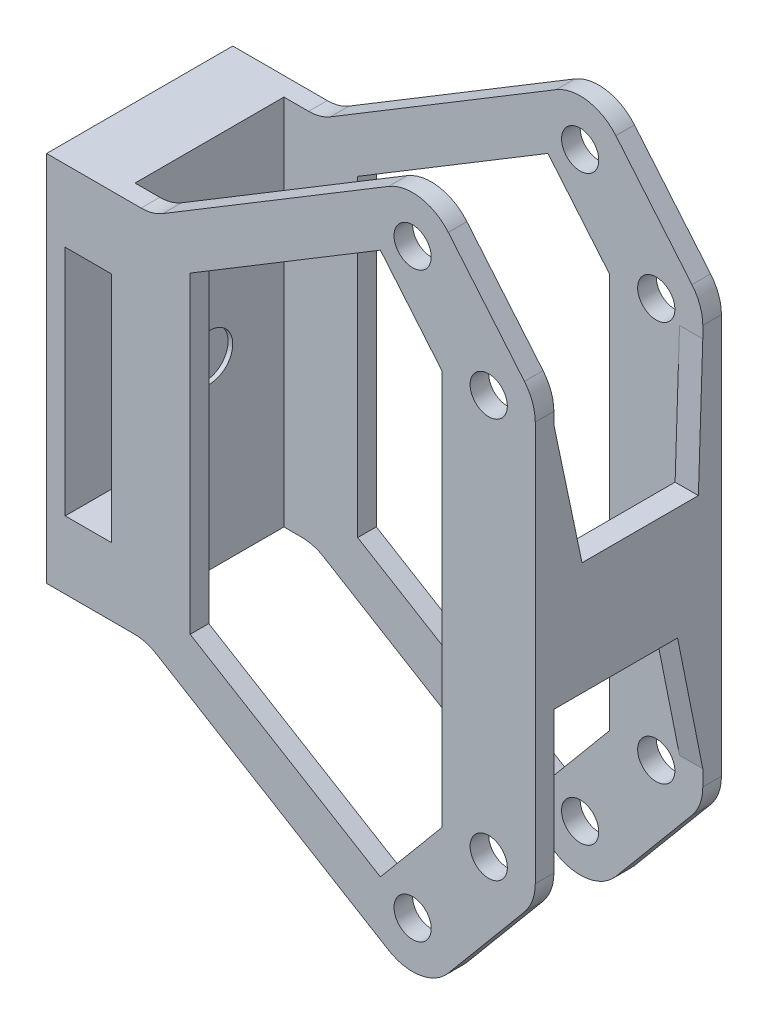
from build123d import *

# Parameters (mm, degrees)
BRACKET_PROFILE_SKETCH_R    = 4
BRACKET_PROFILE_SKETCH_W    = 10
BRACKET_PROFILE_SKETCH_H    = 50
BRACKET_BODY_DEPTH          = 20
SIDE_CUTOUT_DEPTH           = 151.958708937
SIDE_CUTOUT_DEPTH_BACK      = 151.958708937
SIDE_CUTOUT_SKETCH_W        = 85
SIDE_CUTOUT_SKETCH_H        = 32
INNER_WINDOW_CUT_DEPTH      = 130.155913531
INNER_WINDOW_CUT_DEPTH_BACK = 130.155913531
INNER_WINDOW_SKETCH_W       = 32
INNER_WINDOW_SKETCH_H       = 12.117592982
INNER_WINDOW_SKETCH_H_2     = 13.000486956
SIDE_OPENINGS_CUT_DEPTH     = 40
HOLE_10_SKETCH_R            = 5
THROUGH_HOLE_10_DEPTH       = 40
RECESS_24_SKETCH_R          = 12
RECESS_24X3_DEPTH           = 3


with BuildPart() as part:
    # Bracket Profile Sketch → Bracket Body (new, symmetric)
    with BuildSketch(Plane.XY):
        with BuildLine():
            Line((18.112706939, 41.738939357), (66.624129095, 71.058341812))
            ThreePointArc((66.624129095, 71.058341812), (73.442433942, 72.363637042), (79.467576157, 68.915342115))
            Line((79.467576157, 68.915342115), (95.817576157, 49.365342115))
            ThreePointArc((95.817576157, 49.365342115), (97.546351125, 46.362517955), (98.146631916, 42.95))
            Line((98.146631916, 42.95), (98.146631916, -42.95))
            ThreePointArc((98.146631916, -42.95), (97.546351125, -46.362517955), (95.817576157, -49.365342115))
            Line((95.817576157, -49.365342115), (79.467576157, -68.915342115))
            ThreePointArc((79.467576157, -68.915342115), (73.442433942, -72.363637042), (66.624129095, -71.058341812))
            Line((66.624129095, -71.058341812), (16.651884454, -40.856045382))
            ThreePointArc((16.651884454, -40.856045382), (14.412975364, -39.88899222), (11.996631916, -39.558553013))
            Line((11.996631916, -39.558553013), (-6.853368084, -39.558553013))
            Line((-6.853368084, -39.558553013), (-6.853368084, 40.441446987))
            Line((-6.853368084, 40.441446987), (13.4574544, 40.441446987))
            ThreePointArc((13.4574544, 40.441446987), (15.873797849, 40.771886195), (18.112706939, 41.738939357))
        make_face()
        with Locations((88.146631916, 42.95)):
            Circle(BRACKET_PROFILE_SKETCH_R, mode=Mode.SUBTRACT)
        with Locations((71.796631916, 62.5)):
            Circle(BRACKET_PROFILE_SKETCH_R, mode=Mode.SUBTRACT)
        with Locations(Location((88.146631916, -42.95, 0), (0, 0, 180))):
            Circle(BRACKET_PROFILE_SKETCH_R, mode=Mode.SUBTRACT)
        with Locations(Location((71.796631916, -62.5, 0), (0, 0, 180))):
            Circle(BRACKET_PROFILE_SKETCH_R, mode=Mode.SUBTRACT)
        with Locations((2.146631916, 0)):
            Rectangle(BRACKET_PROFILE_SKETCH_W, BRACKET_PROFILE_SKETCH_H, mode=Mode.SUBTRACT)
        Polygon((23.996631916, 33.610567881), (23.996631916, -33.610567881), (64.869180084, -58.31317679), (78.146631916, -42.437079952), (78.146631916, 42.437079952), (64.869180084, 58.31317679), align=None, mode=Mode.SUBTRACT)
    extrude(amount=BRACKET_BODY_DEPTH, both=True)

    # Side Cutout Sketch → Side Cutout (cut, two sides: drawn at the far end of the back side and taken through both)
    with BuildSketch(Plane(origin=(0, 40.441446987, 0), x_dir=(1, 0, 0), z_dir=(0, 1, 0)).offset(-SIDE_CUTOUT_DEPTH_BACK)):
        with Locations((50.646631916, 0)):
            Rectangle(SIDE_CUTOUT_SKETCH_W, SIDE_CUTOUT_SKETCH_H)
    extrude(amount=SIDE_CUTOUT_DEPTH + SIDE_CUTOUT_DEPTH_BACK, mode=Mode.SUBTRACT)

    # Inner Window Sketch → Inner Window Cut (cut, two sides: drawn at the far end of the back side and taken through both)
    with BuildSketch(Plane.ZY.offset(6.853368084).offset(-INNER_WINDOW_CUT_DEPTH_BACK)):
        with Locations((0, 46.500243478)):
            Rectangle(INNER_WINDOW_SKETCH_W, INNER_WINDOW_SKETCH_H)
        with Locations((0, -46.058796491)):
            Rectangle(INNER_WINDOW_SKETCH_W, INNER_WINDOW_SKETCH_H_2)
    extrude(amount=INNER_WINDOW_CUT_DEPTH + INNER_WINDOW_CUT_DEPTH_BACK, mode=Mode.SUBTRACT)

    # Side Openings Sketch → Side Openings Cut (cut)
    with BuildSketch(Plane(origin=(98.146631916, 0, 0), x_dir=(0, 0, -1), z_dir=(1, 0, 0))):
        Polygon((-16, -39.558553013), (-16, -12.5), (10.579626048, -12.5), (16, -39.558553013), align=None)
        Polygon((-16, 40.441446987), (-9.950879321, 11.757125531), (15.049120679, 11.757125531), (16, 40.441446987), align=None)
    extrude(amount=-SIDE_OPENINGS_CUT_DEPTH, mode=Mode.SUBTRACT)

    # Hole Ø10 Sketch → Through Hole Ø10 (cut)
    with BuildSketch(Plane.ZY.offset(6.853368084)):
        Circle(HOLE_10_SKETCH_R)
    extrude(amount=-THROUGH_HOLE_10_DEPTH, mode=Mode.SUBTRACT)

    # Recess Ø24 Sketch → Recess Ø24x3 (cut)
    with BuildSketch(Plane.ZY.offset(6.853368084)):
        Circle(RECESS_24_SKETCH_R)
    extrude(amount=-RECESS_24X3_DEPTH, mode=Mode.SUBTRACT)


solid = part.part
